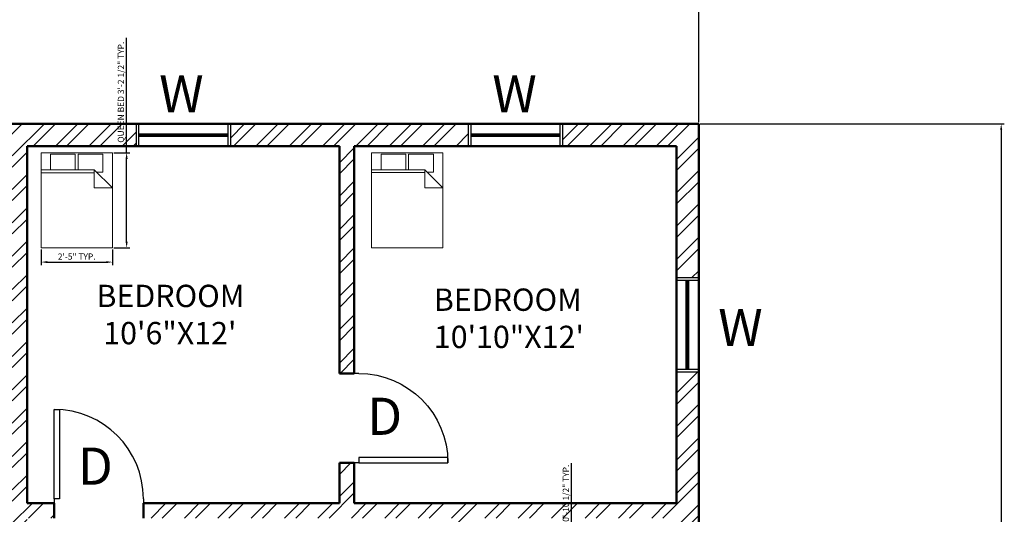
# Model space of a CAD drawing. Units: inches. Extents: x -31485 to -28799, y 18003 to 19130.
# Tile 6 of 15: x -30936 to -30538, y 18666 to 18866. Entities that reach past the tile are written whole.
import ezdxf

# ---------------------------------------------------------------- set-up
doc = ezdxf.new("R2010")
doc.units = ezdxf.units.IN
for name, color, linetype, lineweight in [('A-ANNO-DIMS', 2, 'Continuous', 18), ('A-ANNO-TEXT', 7, 'Continuous', 18), ('A-AREA-IDEN', 7, 'Continuous', 18), ('A-DOOR', 3, 'Continuous', 25), ('A-FURN', 8, 'Continuous', 18), ('A-GLAZ', 4, 'Continuous', 25), ('A-WALL', 7, 'Continuous', 50), ('A-WALL-PATT', 8, 'Continuous', 13)]:
    doc.layers.add(name, color=color, linetype=linetype, lineweight=lineweight)
doc.styles.get("Standard").update_dxf_attribs({"font": 'arial.ttf'})
doc.dimstyles.new('ISO-25', dxfattribs={"dimtxt": 2.5, "dimasz": 2.5, "dimexe": 1.25, "dimexo": 0.625, "dimtad": 1, "dimdec": 0, "dimlunit": 3, "dimtxsty": 'Standard', "dimcen": 2.5, "dimadec": 0, "dimazin": 0, "dimtfac": 1, "dimtdec": 0, "dimtmove": 0, "dimatfit": 3, "dimfxl": 1, "dimarcsym": 0})

# ---------------------------------------------------------------- blocks, each defined once
blk = doc.blocks.new('*U8')
for p, q in [((0, 0), (0, -100)), ((750, 0), (750, -100))]:
    blk.add_line(p, q)
blk.add_lwpolyline([(0, 0), (0, 750), (43.75, 750), (43.75, 0)], close=True)
blk.add_arc((0, 0), 750, 0, 90)
blk = doc.blocks.new('Bed - Queen')
for p, q in [((0, -80.00003), (0, 0)), ((0, 0), (59.99999, 0)), ((59.99999, 0), (59.99999, -80.00003)), ((7.99999, -1.2), (28.79998, -1.2)), ((7.99999, -14.4), (7.99999, -1.2)), ((28.79998, -1.2), (28.79998, -14.4)), ((31.19999, -1.2), (51.99999, -1.2)), ((31.19999, -14.4), (31.19999, -1.2)), ((51.99999, -1.2), (51.99999, -16.4)), ((0, -14.4), (44.8, -14.4)), ((59.99999, -29.6), (44.8, -14.4)), ((44.8, -14.4), (44.8, -29.6)), ((51.99999, -16.4), (46.79936, -16.4)), ((44.8, -16.8), (0, -16.8)), ((44.8, -29.6), (59.99999, -29.6)), ((59.99999, -80.00003), (0, -80.00003))]:
    blk.add_line(p, q)
blk = doc.blocks.new('*D200')
at = {"layer": 'A-ANNO-DIMS', "color": 0, "lineweight": -2, "transparency": 16777216}
for p, q in [((-31209.53, 18824.43), (-31209.53, 18901.41)), ((-31207.03, 18900.16), (-30664.03, 18900.16)), ((-30661.53, 18824.43), (-30661.53, 18901.41))]:
    blk.add_line(p, q, dxfattribs=at)
at = {"layer": 'A-ANNO-DIMS', "color": 0, "transparency": 16777216}
for points in [[(-31207.03, 18900.58), (-31207.03, 18899.75), (-31209.53, 18900.16)], [(-30664.03, 18900.58), (-30664.03, 18899.75), (-30661.53, 18900.16)]]:
    blk.add_solid(points, dxfattribs=at)
at = {"layer": 'Defpoints', "color": 0, "transparency": 16777216}
for p in [(-30661.53, 18900.16), (-31209.53, 18823.8), (-30661.53, 18823.8)]:
    blk.add_point(p, dxfattribs=at)
at = {"layer": 'A-ANNO-DIMS', "color": 0, "transparency": 16777216, "insert": (-30935.53, 18908.96), "char_height": 2.5, "attachment_point": 5}
blk.add_mtext('{\\H6.4x;45\'-8"}', dxfattribs=at)
blk = doc.blocks.new('*D199')
at = {"layer": 'A-ANNO-DIMS', "color": 0, "lineweight": -2, "transparency": 16777216}
for p, q in [((-30660.9, 18823.8), (-30538.22, 18823.8)), ((-30539.47, 18821.3), (-30539.47, 18182.3)), ((-30660.9, 18179.8), (-30538.22, 18179.8))]:
    blk.add_line(p, q, dxfattribs=at)
at = {"layer": 'A-ANNO-DIMS', "color": 0, "transparency": 16777216}
for points in [[(-30539.88, 18821.3), (-30539.05, 18821.3), (-30539.47, 18823.8)], [(-30539.88, 18182.3), (-30539.05, 18182.3), (-30539.47, 18179.8)]]:
    blk.add_solid(points, dxfattribs=at)
at = {"layer": 'Defpoints', "color": 0, "transparency": 16777216}
for p in [(-30661.53, 18823.8), (-30661.53, 18179.8), (-30539.47, 18179.8)]:
    blk.add_point(p, dxfattribs=at)
at = {"layer": 'A-ANNO-DIMS', "color": 0, "transparency": 16777216, "insert": (-30548.27, 18501.8), "char_height": 2.5, "attachment_point": 5, "rotation": 90}
blk.add_mtext('{\\H6.4x;53\'-8"}', dxfattribs=at)
blk = doc.blocks.new('WIN-900-W9')
for p, q in [((-29982.21, 18824.12), (-29982.21, 18815.12)), ((-29981.21, 18824.12), (-29981.21, 18815.12)), ((-29945.21, 18824.12), (-29945.21, 18815.12)), ((-29944.21, 18824.12), (-29944.21, 18815.12)), ((-29981.21, 18820.12), (-29945.21, 18820.12)), ((-29981.21, 18819.62), (-29945.21, 18819.62)), ((-29981.21, 18819.12), (-29945.21, 18819.12))]:
    blk.add_line(p, q)
blk = doc.blocks.new('*D220')
at = {"layer": 'A-ANNO-DIMS', "color": 0, "lineweight": -2, "transparency": 16777216}
for p, q in [((-30892.38, 18812.14), (-30892.38, 18858.49)), ((-30897.51, 18812.14), (-30891.13, 18812.14)), ((-30892.38, 18776.29), (-30892.38, 18809.64)), ((-30897.51, 18773.79), (-30891.13, 18773.79))]:
    blk.add_line(p, q, dxfattribs=at)
at = {"layer": 'A-ANNO-DIMS', "color": 0, "transparency": 16777216}
for points in [[(-30892.8, 18809.64), (-30891.96, 18809.64), (-30892.38, 18812.14)], [(-30892.8, 18776.29), (-30891.96, 18776.29), (-30892.38, 18773.79)]]:
    blk.add_solid(points, dxfattribs=at)
at = {"layer": 'Defpoints', "color": 0, "transparency": 16777216}
for p in [(-30898.13, 18812.14), (-30892.38, 18812.14), (-30898.13, 18773.79)]:
    blk.add_point(p, dxfattribs=at)
at = {"layer": 'A-ANNO-DIMS', "color": 0, "transparency": 16777216, "insert": (-30894.37, 18836.56), "char_height": 2.5, "attachment_point": 5, "rotation": 90}
blk.add_mtext('QUEEN BED 3\'-2 1/2" TYP.', dxfattribs=at)
blk = doc.blocks.new('*D221')
at = {"layer": 'A-ANNO-DIMS', "color": 0, "lineweight": -2, "transparency": 16777216}
for p, q in [((-30926.89, 18773.16), (-30926.89, 18766.79)), ((-30898.13, 18773.16), (-30898.13, 18766.79)), ((-30924.39, 18768.04), (-30900.63, 18768.04))]:
    blk.add_line(p, q, dxfattribs=at)
at = {"layer": 'A-ANNO-DIMS', "color": 0, "transparency": 16777216}
for points in [[(-30924.39, 18768.45), (-30924.39, 18767.62), (-30926.89, 18768.04)], [(-30900.63, 18768.45), (-30900.63, 18767.62), (-30898.13, 18768.04)]]:
    blk.add_solid(points, dxfattribs=at)
at = {"layer": 'Defpoints', "color": 0, "transparency": 16777216}
for p in [(-30926.89, 18773.79), (-30898.13, 18773.79), (-30898.13, 18768.04)]:
    blk.add_point(p, dxfattribs=at)
at = {"layer": 'A-ANNO-DIMS', "color": 0, "transparency": 16777216, "insert": (-30912.51, 18769.94), "char_height": 2.5, "attachment_point": 5}
blk.add_mtext('2\'-5" TYP.', dxfattribs=at)
blk = doc.blocks.new('*D249')
at = {"layer": 'A-ANNO-DIMS', "color": 0, "lineweight": -2, "transparency": 16777216}
for p, q in [((-30712.9, 18660.18), (-30712.9, 18686.94)), ((-30714.07, 18660.18), (-30711.65, 18660.18)), ((-30712.9, 18652.28), (-30712.9, 18657.68)), ((-30714.07, 18649.78), (-30711.65, 18649.78))]:
    blk.add_line(p, q, dxfattribs=at)
at = {"layer": 'A-ANNO-DIMS', "color": 0, "transparency": 16777216}
for points in [[(-30713.31, 18657.68), (-30712.48, 18657.68), (-30712.9, 18660.18)], [(-30713.31, 18652.28), (-30712.48, 18652.28), (-30712.9, 18649.78)]]:
    blk.add_solid(points, dxfattribs=at)
at = {"layer": 'Defpoints', "color": 0, "transparency": 16777216}
for p in [(-30714.7, 18660.18), (-30712.9, 18660.18), (-30714.7, 18649.78)]:
    blk.add_point(p, dxfattribs=at)
at = {"layer": 'A-ANNO-DIMS', "color": 0, "transparency": 16777216, "insert": (-30714.82, 18674.81), "char_height": 2.5, "attachment_point": 5, "rotation": 90}
blk.add_mtext('0\'-10 1/2" TYP.', dxfattribs=at)

msp = doc.modelspace()

# ---------------------------------------------------------------- hatches: boundary and pattern name
at = {"layer": 'A-WALL-PATT'}
h = msp.add_hatch(dxfattribs=at)
h.set_pattern_fill('ANSI32', color=256)
h.set_pattern_definition([(45, (-1687.357, -0.313), (-6.735192, 6.735192), []), (45, (-1682.867, -0.313), (-6.735192, 6.735192), [])])
h.paths.add_polyline_path([(-31156.53, 18823.8), (-31209.53, 18823.8), (-31209.53, 18761.8), (-31200.53, 18761.8), (-31200.53, 18814.8), (-31156.53, 18814.8)], flags=17)
h.paths.add_polyline_path([(-31022.53, 18823.8), (-31118.53, 18823.8), (-31118.53, 18814.8), (-31074.53, 18814.8), (-31074.53, 18720.79), (-31070.96, 18720.79), (-31068.53, 18720.76), (-31068.53, 18814.8), (-31022.53, 18814.8)], flags=17)
h.paths.add_polyline_path([(-30754.53, 18823.8), (-30850.53, 18823.8), (-30850.53, 18814.8), (-30806.53, 18814.8), (-30806.53, 18723.1), (-30800.53, 18723.1), (-30800.53, 18814.8), (-30754.53, 18814.8)], flags=17)
h.paths.add_polyline_path([(-30661.53, 18823.8), (-30716.53, 18823.8), (-30716.53, 18814.8), (-30670.53, 18814.8), (-30670.53, 18761.8), (-30661.53, 18761.8)], flags=17)
h.paths.add_polyline_path([(-30986.92, 18670.8), (-31068.53, 18670.8), (-31068.53, 18684.76), (-31074.53, 18684.76), (-31074.53, 18670.8), (-31200.53, 18670.8), (-31200.53, 18723.8), (-31209.53, 18723.8), (-31209.53, 18641.8), (-31200.53, 18641.8), (-31200.53, 18664.8), (-31104.53, 18664.8), (-31104.53, 18628.93), (-31098.53, 18628.93), (-31098.53, 18664.8), (-30986.92, 18664.8)], flags=17)
h.paths.add_polyline_path([(-30661.53, 18723.8), (-30670.53, 18723.8), (-30670.53, 18670.8), (-30800.53, 18670.8), (-30800.53, 18687.1), (-30806.53, 18687.1), (-30806.53, 18670.8), (-30885.6, 18670.8), (-30885.6, 18667.8), (-30885.6, 18664.8), (-30760.53, 18664.8), (-30760.53, 18625.8), (-30754.53, 18625.8), (-30754.53, 18664.8), (-30670.53, 18664.8), (-30670.53, 18641.8), (-30661.53, 18641.8)], flags=17)
h.paths.add_polyline_path([(-31200.53, 18574.8), (-31188.56, 18574.8), (-31188.56, 18580.8), (-31200.53, 18580.8), (-31200.53, 18603.8), (-31209.53, 18603.8), (-31209.53, 18557.8), (-31200.53, 18557.8)], flags=17)
h.paths.add_polyline_path([(-31098.53, 18592.93), (-31104.53, 18592.93), (-31104.53, 18580.8), (-31164.56, 18580.8), (-31164.56, 18574.8), (-31104.53, 18574.8), (-31104.53, 18514.8), (-31200.53, 18514.8), (-31200.53, 18531.8), (-31209.53, 18531.8), (-31209.53, 18473.8), (-31200.53, 18473.8), (-31200.53, 18508.8), (-31056.53, 18508.8), (-31056.53, 18501.62), (-31050.53, 18501.62), (-31050.53, 18514.8), (-31098.53, 18514.8)], flags=17)
h.paths.add_polyline_path([(-30661.53, 18531.8), (-30670.53, 18531.8), (-30670.53, 18514.8), (-30754.53, 18514.8), (-30754.53, 18574.8), (-30700.75, 18574.8), (-30700.75, 18577.44), (-30700.75, 18580.8), (-30754.53, 18580.8), (-30754.53, 18589.8), (-30760.53, 18589.8), (-30760.53, 18514.8), (-30820.53, 18514.8), (-30820.53, 18499.26), (-30814.53, 18499.26), (-30814.53, 18508.8), (-30670.53, 18508.8), (-30670.53, 18473.8), (-30661.53, 18473.8)], flags=17)
h.paths.add_polyline_path([(-30661.53, 18435.8), (-30670.53, 18435.8), (-30670.53, 18400.8), (-30814.53, 18400.8), (-30814.53, 18413.15), (-30820.53, 18413.15), (-30820.53, 18400.8), (-30932.53, 18400.8), (-30932.53, 18664.8), (-30921.6, 18664.8), (-30921.6, 18670.8), (-30932.53, 18670.8), (-30932.53, 18814.8), (-30888.53, 18814.8), (-30888.53, 18823.8), (-30984.53, 18823.8), (-30984.53, 18814.8), (-30938.53, 18814.8), (-30938.53, 18670.8), (-30950.92, 18670.8), (-30950.92, 18664.8), (-30938.53, 18664.8), (-30938.53, 18400.8), (-31050.53, 18400.8), (-31050.53, 18411.18), (-31056.53, 18411.18), (-31056.53, 18400.8), (-31200.53, 18400.8), (-31200.53, 18435.8), (-31209.53, 18435.8), (-31209.53, 18179.8), (-31200.53, 18179.8), (-31200.53, 18394.8), (-31001.53, 18394.8), (-31001.53, 18179.8), (-30954.53, 18179.8), (-30954.53, 18188.8), (-30995.53, 18188.8), (-30995.53, 18394.8), (-30875.53, 18394.8), (-30875.53, 18188.8), (-30916.53, 18188.8), (-30916.53, 18179.8), (-30869.53, 18179.8), (-30869.53, 18394.8), (-30670.53, 18394.8), (-30670.53, 18179.8), (-30661.53, 18179.8)])

# ---------------------------------------------------------------- linework, layer by layer
at = {"layer": 'A-WALL'}
for p, q in [((-31209.53, 18823.8), (-30661.53, 18823.8)), ((-30661.53, 18823.8), (-30661.53, 18179.8)), ((-30932.53, 18814.8), (-30806.53, 18814.8)), ((-30932.53, 18814.8), (-30932.53, 18670.8)), ((-30806.53, 18814.8), (-30806.53, 18723.1)), ((-30800.53, 18814.8), (-30670.53, 18814.8)), ((-30800.53, 18814.8), (-30800.53, 18723.1)), ((-30670.53, 18814.8), (-30670.53, 18670.8)), ((-30806.53, 18723.1), (-30800.53, 18723.1)), ((-30806.53, 18687.1), (-30806.53, 18670.8)), ((-30806.53, 18687.1), (-30800.53, 18687.1)), ((-30800.53, 18687.1), (-30800.53, 18670.8)), ((-30932.53, 18670.8), (-30921.6, 18670.8)), ((-30921.6, 18670.8), (-30921.6, 18664.8)), ((-30885.6, 18670.8), (-30806.53, 18670.8)), ((-30885.6, 18670.8), (-30885.6, 18664.8)), ((-30800.53, 18670.8), (-30670.53, 18670.8))]:
    msp.add_line(p, q, dxfattribs=at)

# ---------------------------------------------------------------- block references
at = {"layer": 'A-DOOR', "xscale": -0.0479999995519333, "yscale": 0.0479999995519333, "zscale": 0.0479999995519333, "rotation": 270}
msp.add_blockref('*U8', (-30798.73, 18687.1), dxfattribs=at)
at = {"layer": 'A-DOOR', "xscale": 0.0480000000000013, "yscale": 0.0480000000000013, "zscale": 0.0480000000000013}
msp.add_blockref('*U8', (-30921.6, 18672.6), dxfattribs=at)
at = {"layer": 'A-FURN', "xscale": 0.479364226334794, "yscale": 0.479364226334794, "zscale": 0.479364226334794}
for p in [(-30926.89, 18812.14), (-30793.54, 18812.17)]:
    msp.add_blockref('Bed - Queen', p, dxfattribs=at)
at = {"layer": 'A-GLAZ'}
for p in [(-906.32, -0.31), (-772.32, -0.31)]:
    msp.add_blockref('WIN-900-W9', p, dxfattribs=at)
at = {"layer": 'A-GLAZ', "rotation": 89.99999999997677}
msp.add_blockref('WIN-900-W9', (-11846.41, 48706.01), dxfattribs=at)

# ---------------------------------------------------------------- texts
at = {"layer": 'A-ANNO-TEXT', "char_height": 15, "attachment_point": 1}
for s, insert in [('{W}', (-30879.26, 18843.38)), ('{W}', (-30744.82, 18843.38)), ('{W}', (-30653.67, 18749.17)), ('{D}', (-30795.3, 18713.33)), ('{D}', (-30912.03, 18693.22))]:
    msp.add_mtext_dynamic_manual_height_columns(s, width=638.549, gutter_width=12.5, heights=[0], dxfattribs=dict(at, insert=insert))
at = {"layer": 'A-AREA-IDEN', "char_height": 9, "attachment_point": 1}
for s, insert in [('{BEDROOM\\P 10\'6"X12\'}', (-30904.56, 18758.89)), ('{ BEDROOM\\P 10\'10"X12\'}', (-30771.17, 18757.37))]:
    msp.add_mtext_dynamic_manual_height_columns(s, width=763.1479, gutter_width=12.5, heights=[0], dxfattribs=dict(at, insert=insert))

# ---------------------------------------------------------------- dimensions: what is measured, and where the dimension line sits
at = {"layer": 'A-ANNO-DIMS'}
for base, p1, p2, text, override, picture, middle in [((-30661.53, 18900.16), (-31209.53, 18823.8), (-30661.53, 18823.8), '{\\H6.4x;<>}', {"dimclrd": 0, "dimclre": 0, "dimclrt": 0}, '*D200', (-30935.53, 18908.96)), ((-30898.13, 18768.04), (-30926.89, 18773.79), (-30898.13, 18773.79), '<> TYP.', {"dimdec": 1, "dimlfac": 1, "dimrnd": 0, "dimzin": 1, "dimdsep": 46, "dimlunit": 4, "dimfrac": 2}, '*D221', (-30912.51, 18769.94))]:
    dim = msp.add_linear_dim(base=base, p1=p1, p2=p2, text=text, dimstyle='ISO-25', override=override, dxfattribs=at)
    dim.commit()
    dim.dimension.update_dxf_attribs({"geometry": picture, "text_midpoint": middle})
for base, p1, p2, text, override, picture, middle in [((-30892.3786, 18812.1373), (-30898.131, 18773.7882), (-30898.131, 18812.1373), 'QUEEN BED <> TYP.', {"dimdec": 1, "dimlfac": 1, "dimrnd": 0, "dimzin": 1, "dimdsep": 46, "dimlunit": 4, "dimfrac": 2}, '*D220', (-30894.373, 18836.5626)), ((-30539.47, 18179.8), (-30661.53, 18823.8), (-30661.53, 18179.8), '{\\H6.4x;<>}', {"dimclrd": 0, "dimclre": 0, "dimclrt": 0}, '*D199', (-30548.27, 18501.8)), ((-30712.9, 18660.18), (-30714.7, 18649.78), (-30714.7, 18660.18), '<> TYP.', {"dimdec": 1, "dimlfac": 1, "dimrnd": 0, "dimzin": 1, "dimdsep": 46, "dimlunit": 4, "dimfrac": 2}, '*D249', (-30714.82, 18674.81))]:
    dim = msp.add_linear_dim(base=base, p1=p1, p2=p2, angle=90, text=text, dimstyle='ISO-25', override=override, dxfattribs=at)
    dim.commit()
    dim.dimension.update_dxf_attribs({"geometry": picture, "text_midpoint": middle})

doc.saveas('drawing.dxf')
